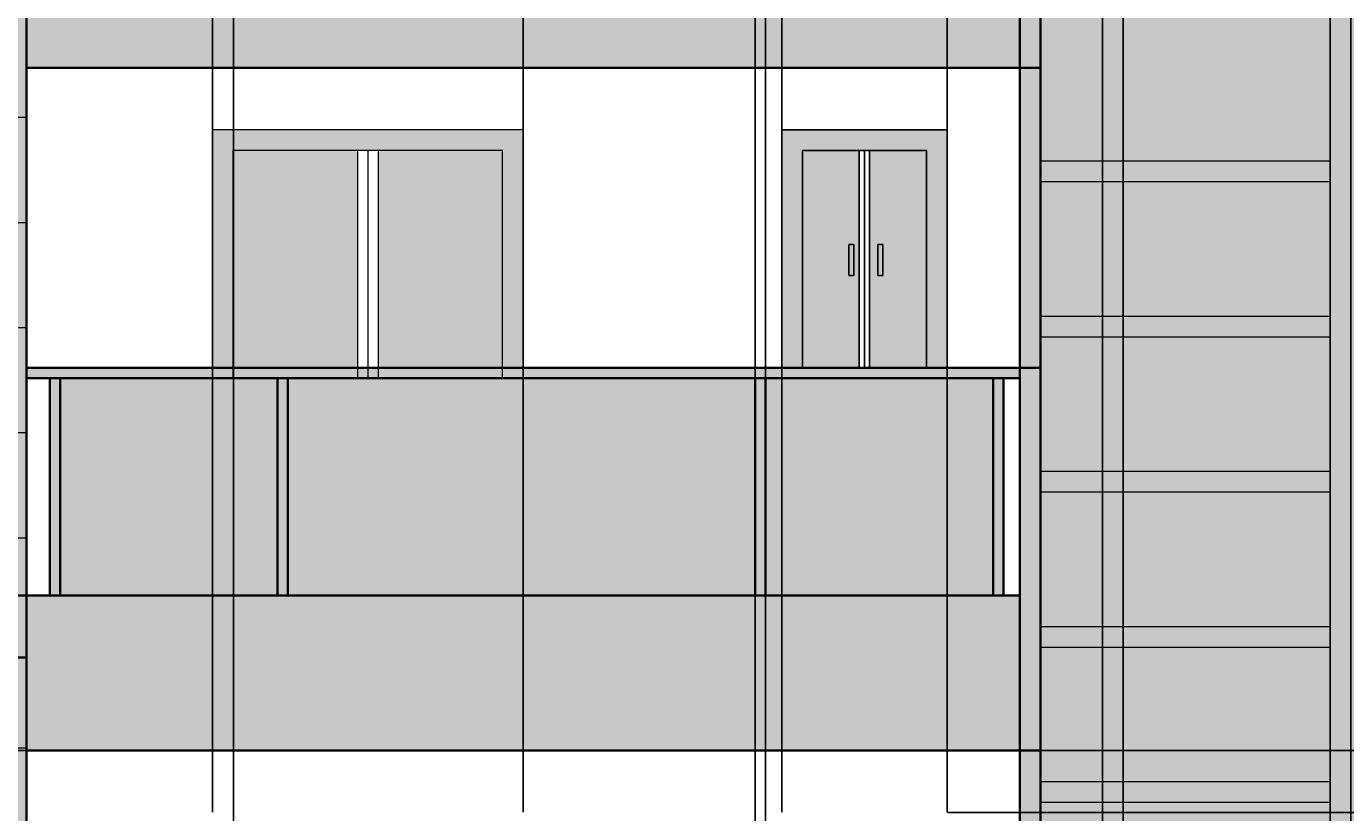
# Model space of a CAD drawing. Units: inches. Extents: x 2794 to 3619, y 522 to 1397.
# Tile 4 of 10: x 2954 to 3209, y 821 to 973. Entities that reach past the tile are written whole.
import ezdxf

# ---------------------------------------------------------------- set-up
doc = ezdxf.new("R2010")
doc.units = ezdxf.units.IN
for name, color, linetype, lineweight in [('A-ANNO-DIMS', 2, 'Continuous', 18), ('A-DOOR', 3, 'Continuous', 25), ('A-ELEV', 7, 'Continuous', 35), ('A-ELEV-PATT', 8, 'Continuous', 13), ('A-GLAZ', 4, 'Continuous', 18)]:
    doc.layers.add(name, color=color, linetype=linetype, lineweight=lineweight)
doc.styles.get("Standard").update_dxf_attribs({"font": 'arial.ttf'})
doc.dimstyles.get("Standard").update_dxf_attribs({"dimtxt": 0.18, "dimasz": 0.18, "dimexe": 0.18, "dimexo": 0.0625, "dimgap": 0.09, "dimtad": 0, "dimtih": 1, "dimtoh": 1, "dimdec": 4, "dimzin": 0, "dimdsep": 46, "dimtxsty": 'Standard', "dimcen": 0.09, "dimadec": 0, "dimazin": 0, "dimtfac": 1, "dimtdec": 4, "dimtofl": 0, "dimtmove": 0, "dimatfit": 3, "dimfxl": 1, "dimtolj": 1, "dimtzin": 0, "dimarcsym": 0})

# ---------------------------------------------------------------- blocks, each defined once
blk = doc.blocks.new('WIN-1500')
at = {"transparency": 33554646}
h = blk.add_hatch(color=256, dxfattribs=at)
h.dxf.hatch_style = 1
h.paths.add_polyline_path([(60, 48), (0, 48), (0, 2), (4, 2), (4, 44), (56, 44), (56, 2), (60, 2)])
at = {"transparency": 33554687}
h = blk.add_hatch(color=256, dxfattribs=at)
h.dxf.hatch_style = 1
h.set_gradient(color1=(248, 246, 176), color2=(74, 13, 14), name='INVCYLINDER')
h.paths.add_polyline_path([(56, 44), (32, 44), (32, 2), (56, 2)])
h.paths.add_polyline_path([(28, 44), (4, 44), (4, 2), (28, 2)])
for p, q in [((0, 0), (0, 48)), ((60, 48), (0, 48)), ((60, 0), (60, 48)), ((56, 44), (4, 44)), ((4, 0), (4, 44)), ((28, 44), (28, 0)), ((30, 44), (30, 0)), ((32, 44), (32, 0)), ((56, 0), (56, 44))]:
    blk.add_line(p, q)
blk = doc.blocks.new('DOOR-BALCONY-DBL')
at = {"transparency": 33554628}
h = blk.add_hatch(color=256, dxfattribs=at)
h.dxf.hatch_style = 1
h.paths.add_polyline_path([(4, 42), (28, 42), (28, 0), (32, 0), (32, 46), (0, 46), (0, 0), (4, 0)])
at = {"transparency": 33554646}
h = blk.add_hatch(color=256, dxfattribs=at)
h.dxf.hatch_style = 1
h.set_gradient(color1=(255, 255, 255), color2=(147, 149, 152), name='INVCYLINDER')
h.paths.add_polyline_path([(15, 42), (4, 42), (4, 0), (15, 0)])
h = blk.add_hatch(color=256, dxfattribs=at)
h.dxf.hatch_style = 1
h.set_gradient(color1=(255, 255, 255), color2=(147, 149, 152), name='INVCYLINDER')
h.paths.add_polyline_path([(28, 42), (17, 42), (17, 0), (28, 0)])
for p, q in [((0, 0), (0, 46)), ((0, 46), (32, 46)), ((4, 46), (28, 46)), ((32, 0), (32, 46)), ((4, 0), (4, 42)), ((4, 42), (28, 42)), ((15, 0), (15, 42)), ((16, 0), (16, 42)), ((17, 0), (17, 42)), ((28, 0), (28, 42))]:
    blk.add_line(p, q)
for points in [[(12.99, 23.83), (13.93, 23.83), (13.93, 17.87), (12.99, 17.87)], [(18.59, 23.83), (19.53, 23.83), (19.53, 17.87), (18.59, 17.87)]]:
    blk.add_lwpolyline(points, close=True)
blk = doc.blocks.new('*D16')
at = {"layer": 'A-ANNO-DIMS', "color": 0, "lineweight": -2, "transparency": 16777216}
for p, q in [((3142.2, 1356.64), (2793.99, 1356.64)), ((2794.17, 1356.46), (2794.17, 959.82)), ((2794.17, 562.82), (2794.17, 959.45)), ((2834.2, 562.64), (2793.99, 562.64))]:
    blk.add_line(p, q, dxfattribs=at)
at = {"layer": 'A-ANNO-DIMS', "color": 0, "transparency": 16777216}
for points in [[(2794.14, 1356.46), (2794.2, 1356.46), (2794.17, 1356.64)], [(2794.14, 562.82), (2794.2, 562.82), (2794.17, 562.64)]]:
    blk.add_solid(points, dxfattribs=at)
at = {"layer": 'Defpoints', "color": 0, "transparency": 16777216}
for p in [(2794.17, 1356.64), (3142.27, 1356.64), (2834.27, 562.64)]:
    blk.add_point(p, dxfattribs=at)
at = {"layer": 'A-ANNO-DIMS', "color": 0, "transparency": 16777216, "insert": (2794.17, 959.64), "char_height": 0.18, "attachment_point": 5}
blk.add_mtext('\\A1;794', dxfattribs=at)
blk = doc.blocks.new('*D28')
at = {"layer": 'A-ANNO-DIMS', "color": 0, "lineweight": -2, "transparency": 16777216}
for p, q in [((2954.27, 832.7), (2954.27, 1396.92)), ((2954.45, 1396.74), (2972.05, 1396.74)), ((2990.09, 1396.74), (2972.48, 1396.74)), ((2990.27, 820.7), (2990.27, 1396.92))]:
    blk.add_line(p, q, dxfattribs=at)
at = {"layer": 'A-ANNO-DIMS', "color": 0, "transparency": 16777216}
for points in [[(2954.45, 1396.77), (2954.45, 1396.71), (2954.27, 1396.74)], [(2990.09, 1396.77), (2990.09, 1396.71), (2990.27, 1396.74)]]:
    blk.add_solid(points, dxfattribs=at)
at = {"layer": 'Defpoints', "color": 0, "transparency": 16777216}
for p in [(2990.27, 1396.74), (2954.27, 832.64), (2990.27, 820.64)]:
    blk.add_point(p, dxfattribs=at)
at = {"layer": 'A-ANNO-DIMS', "color": 0, "transparency": 16777216, "insert": (2972.27, 1396.74), "char_height": 0.18, "attachment_point": 5}
blk.add_mtext('\\A1;36', dxfattribs=at)
blk = doc.blocks.new('*D29')
at = {"layer": 'A-ANNO-DIMS', "color": 0, "lineweight": -2, "transparency": 16777216}
for p, q in [((2990.27, 820.7), (2990.27, 1396.92)), ((2990.45, 1396.74), (2992.11, 1396.74)), ((2994.09, 1396.74), (2992.42, 1396.74)), ((2994.27, 816.7), (2994.27, 1396.92))]:
    blk.add_line(p, q, dxfattribs=at)
at = {"layer": 'A-ANNO-DIMS', "color": 0, "transparency": 16777216}
for points in [[(2990.45, 1396.77), (2990.45, 1396.71), (2990.27, 1396.74)], [(2994.09, 1396.77), (2994.09, 1396.71), (2994.27, 1396.74)]]:
    blk.add_solid(points, dxfattribs=at)
at = {"layer": 'Defpoints', "color": 0, "transparency": 16777216}
for p in [(2994.27, 1396.74), (2990.27, 820.64), (2994.27, 816.64)]:
    blk.add_point(p, dxfattribs=at)
at = {"layer": 'A-ANNO-DIMS', "color": 0, "transparency": 16777216, "insert": (2992.27, 1396.74), "char_height": 0.18, "attachment_point": 5}
blk.add_mtext('\\A1;4', dxfattribs=at)
blk = doc.blocks.new('*D30')
at = {"layer": 'A-ANNO-DIMS', "color": 0, "lineweight": -2, "transparency": 16777216}
for p, q in [((3050.27, 820.7), (3050.27, 1396.92)), ((3050.45, 1396.74), (3075.05, 1396.74)), ((3100.09, 1396.74), (3075.48, 1396.74)), ((3100.27, 820.7), (3100.27, 1396.92))]:
    blk.add_line(p, q, dxfattribs=at)
at = {"layer": 'A-ANNO-DIMS', "color": 0, "transparency": 16777216}
for points in [[(3050.45, 1396.77), (3050.45, 1396.71), (3050.27, 1396.74)], [(3100.09, 1396.77), (3100.09, 1396.71), (3100.27, 1396.74)]]:
    blk.add_solid(points, dxfattribs=at)
at = {"layer": 'Defpoints', "color": 0, "transparency": 16777216}
for p in [(3100.27, 1396.74), (3050.27, 820.64), (3100.27, 820.64)]:
    blk.add_point(p, dxfattribs=at)
at = {"layer": 'A-ANNO-DIMS', "color": 0, "transparency": 16777216, "insert": (3075.27, 1396.74), "char_height": 0.18, "attachment_point": 5}
blk.add_mtext('\\A1;50', dxfattribs=at)
blk = doc.blocks.new('*D31')
at = {"layer": 'A-ANNO-DIMS', "color": 0, "lineweight": -2, "transparency": 16777216}
for p, q in [((3132.27, 820.7), (3132.27, 1396.92)), ((3132.45, 1396.74), (3139.06, 1396.74)), ((3146.09, 1396.74), (3139.48, 1396.74)), ((3146.27, 774.7), (3146.27, 1396.92))]:
    blk.add_line(p, q, dxfattribs=at)
at = {"layer": 'A-ANNO-DIMS', "color": 0, "transparency": 16777216}
for points in [[(3132.45, 1396.77), (3132.45, 1396.71), (3132.27, 1396.74)], [(3146.09, 1396.77), (3146.09, 1396.71), (3146.27, 1396.74)]]:
    blk.add_solid(points, dxfattribs=at)
at = {"layer": 'Defpoints', "color": 0, "transparency": 16777216}
for p in [(3146.27, 1396.74), (3132.27, 820.64), (3146.27, 774.64)]:
    blk.add_point(p, dxfattribs=at)
at = {"layer": 'A-ANNO-DIMS', "color": 0, "transparency": 16777216, "insert": (3139.27, 1396.74), "char_height": 0.18, "attachment_point": 5}
blk.add_mtext('\\A1;14', dxfattribs=at)
blk = doc.blocks.new('*D37')
at = {"layer": 'A-ANNO-DIMS', "color": 0, "lineweight": -2, "transparency": 16777216}
for p, q in [((3095.13, 772.7), (3095.13, 1396.92)), ((3095.31, 1396.74), (3095.98, 1396.74)), ((3096.95, 1396.74), (3096.28, 1396.74)), ((3097.13, 772.7), (3097.13, 1396.92))]:
    blk.add_line(p, q, dxfattribs=at)
at = {"layer": 'A-ANNO-DIMS', "color": 0, "transparency": 16777216}
for points in [[(3095.31, 1396.77), (3095.31, 1396.71), (3095.13, 1396.74)], [(3096.95, 1396.77), (3096.95, 1396.71), (3097.13, 1396.74)]]:
    blk.add_solid(points, dxfattribs=at)
at = {"layer": 'Defpoints', "color": 0, "transparency": 16777216}
for p in [(3097.13, 1396.74), (3095.13, 772.64), (3097.13, 772.64)]:
    blk.add_point(p, dxfattribs=at)
at = {"layer": 'A-ANNO-DIMS', "color": 0, "transparency": 16777216, "insert": (3096.13, 1396.74), "char_height": 0.18, "attachment_point": 5}
blk.add_mtext('\\A1;2', dxfattribs=at)
blk = doc.blocks.new('*D42')
at = {"layer": 'A-ANNO-DIMS', "color": 0, "lineweight": -2, "transparency": 16777216}
for p, q in [((2958.76, 862.64), (2793.99, 862.64)), ((2794.17, 862.46), (2794.17, 847.82)), ((2794.17, 832.82), (2794.17, 847.45)), ((2954.2, 832.64), (2793.99, 832.64))]:
    blk.add_line(p, q, dxfattribs=at)
at = {"layer": 'A-ANNO-DIMS', "color": 0, "transparency": 16777216}
for points in [[(2794.14, 862.46), (2794.2, 862.46), (2794.17, 862.64)], [(2794.14, 832.82), (2794.2, 832.82), (2794.17, 832.64)]]:
    blk.add_solid(points, dxfattribs=at)
at = {"layer": 'Defpoints', "color": 0, "transparency": 16777216}
for p in [(2794.17, 862.64), (2958.83, 862.64), (2954.27, 832.64)]:
    blk.add_point(p, dxfattribs=at)
at = {"layer": 'A-ANNO-DIMS', "color": 0, "transparency": 16777216, "insert": (2794.17, 847.64), "char_height": 0.18, "attachment_point": 5}
blk.add_mtext('\\A1;30', dxfattribs=at)
blk = doc.blocks.new('*D43')
at = {"layer": 'A-ANNO-DIMS', "color": 0, "lineweight": -2, "transparency": 16777216}
for p, q in [((3150.33, 832.64), (3618.55, 832.64)), ((3618.37, 832.46), (3618.37, 826.82)), ((3618.37, 820.82), (3618.37, 826.45)), ((3132.33, 820.64), (3618.55, 820.64))]:
    blk.add_line(p, q, dxfattribs=at)
at = {"layer": 'A-ANNO-DIMS', "color": 0, "transparency": 16777216}
for points in [[(3618.34, 832.46), (3618.4, 832.46), (3618.37, 832.64)], [(3618.34, 820.82), (3618.4, 820.82), (3618.37, 820.64)]]:
    blk.add_solid(points, dxfattribs=at)
at = {"layer": 'Defpoints', "color": 0, "transparency": 16777216}
for p in [(3150.27, 832.64), (3618.37, 832.64), (3132.27, 820.64)]:
    blk.add_point(p, dxfattribs=at)
at = {"layer": 'A-ANNO-DIMS', "color": 0, "transparency": 16777216, "insert": (3618.37, 826.64), "char_height": 0.18, "attachment_point": 5}
blk.add_mtext('\\A1;12', dxfattribs=at)
blk = doc.blocks.new('*D49')
at = {"layer": 'A-ANNO-DIMS', "color": 0, "lineweight": -2, "transparency": 16777216}
for p, q in [((3146.27, 1256.19), (3146.27, 522.36)), ((3150.27, 1254.57), (3150.27, 522.36)), ((3146.45, 522.54), (3148.11, 522.54)), ((3150.09, 522.54), (3148.42, 522.54))]:
    blk.add_line(p, q, dxfattribs=at)
at = {"layer": 'A-ANNO-DIMS', "color": 0, "transparency": 16777216}
for points in [[(3146.45, 522.57), (3146.45, 522.51), (3146.27, 522.54)], [(3150.09, 522.57), (3150.09, 522.51), (3150.27, 522.54)]]:
    blk.add_solid(points, dxfattribs=at)
at = {"layer": 'Defpoints', "color": 0, "transparency": 16777216}
for p in [(3146.27, 1256.25), (3150.27, 1254.64), (3150.27, 522.54)]:
    blk.add_point(p, dxfattribs=at)
at = {"layer": 'A-ANNO-DIMS', "color": 0, "transparency": 16777216, "insert": (3148.27, 522.54), "char_height": 0.18, "attachment_point": 5}
blk.add_mtext('\\A1;4', dxfattribs=at)
blk = doc.blocks.new('*D50')
at = {"layer": 'A-ANNO-DIMS', "color": 0, "lineweight": -2, "transparency": 16777216}
for p, q in [((3150.27, 1254.57), (3150.27, 522.36)), ((3206.27, 1254.57), (3206.27, 522.36)), ((3150.45, 522.54), (3178.05, 522.54)), ((3206.09, 522.54), (3178.48, 522.54))]:
    blk.add_line(p, q, dxfattribs=at)
at = {"layer": 'A-ANNO-DIMS', "color": 0, "transparency": 16777216}
for points in [[(3150.45, 522.57), (3150.45, 522.51), (3150.27, 522.54)], [(3206.09, 522.57), (3206.09, 522.51), (3206.27, 522.54)]]:
    blk.add_solid(points, dxfattribs=at)
at = {"layer": 'Defpoints', "color": 0, "transparency": 16777216}
for p in [(3150.27, 1254.64), (3206.27, 1254.64), (3206.27, 522.54)]:
    blk.add_point(p, dxfattribs=at)
at = {"layer": 'A-ANNO-DIMS', "color": 0, "transparency": 16777216, "insert": (3178.27, 522.54), "char_height": 0.18, "attachment_point": 5}
blk.add_mtext('\\A1;56', dxfattribs=at)
blk = doc.blocks.new('*D51')
at = {"layer": 'A-ANNO-DIMS', "color": 0, "lineweight": -2, "transparency": 16777216}
for p, q in [((3206.27, 1254.57), (3206.27, 522.36)), ((3210.27, 1254.57), (3210.27, 522.36)), ((3206.45, 522.54), (3208.11, 522.54)), ((3210.09, 522.54), (3208.42, 522.54))]:
    blk.add_line(p, q, dxfattribs=at)
at = {"layer": 'A-ANNO-DIMS', "color": 0, "transparency": 16777216}
for points in [[(3206.45, 522.57), (3206.45, 522.51), (3206.27, 522.54)], [(3210.09, 522.57), (3210.09, 522.51), (3210.27, 522.54)]]:
    blk.add_solid(points, dxfattribs=at)
at = {"layer": 'Defpoints', "color": 0, "transparency": 16777216}
for p in [(3206.27, 1254.64), (3210.27, 1254.64), (3210.27, 522.54)]:
    blk.add_point(p, dxfattribs=at)
at = {"layer": 'A-ANNO-DIMS', "color": 0, "transparency": 16777216, "insert": (3208.27, 522.54), "char_height": 0.18, "attachment_point": 5}
blk.add_mtext('\\A1;4', dxfattribs=at)
blk = doc.blocks.new('*D56')
at = {"layer": 'A-ANNO-DIMS', "color": 0, "lineweight": -2, "transparency": 16777216}
for p, q in [((3162.27, 664.7), (3162.27, 1396.92)), ((3162.45, 1396.74), (3206.05, 1396.74)), ((3250.09, 1396.74), (3206.49, 1396.74)), ((3250.27, 664.7), (3250.27, 1396.92))]:
    blk.add_line(p, q, dxfattribs=at)
at = {"layer": 'A-ANNO-DIMS', "color": 0, "transparency": 16777216}
for points in [[(3162.45, 1396.77), (3162.45, 1396.71), (3162.27, 1396.74)], [(3250.09, 1396.77), (3250.09, 1396.71), (3250.27, 1396.74)]]:
    blk.add_solid(points, dxfattribs=at)
at = {"layer": 'Defpoints', "color": 0, "transparency": 16777216}
for p in [(3250.27, 1396.74), (3162.27, 664.64), (3250.27, 664.64)]:
    blk.add_point(p, dxfattribs=at)
at = {"layer": 'A-ANNO-DIMS', "color": 0, "transparency": 16777216, "insert": (3206.27, 1396.74), "char_height": 0.18, "attachment_point": 5}
blk.add_mtext('\\A1;88', dxfattribs=at)
blk = doc.blocks.new('*D57')
at = {"layer": 'A-ANNO-DIMS', "color": 0, "lineweight": -2, "transparency": 16777216}
for p, q in [((3162.27, 664.7), (3162.27, 1396.92)), ((3162.45, 1396.74), (3164.11, 1396.74)), ((3166.09, 1396.74), (3164.42, 1396.74)), ((3166.27, 660.7), (3166.27, 1396.92))]:
    blk.add_line(p, q, dxfattribs=at)
at = {"layer": 'A-ANNO-DIMS', "color": 0, "transparency": 16777216}
for points in [[(3162.45, 1396.77), (3162.45, 1396.71), (3162.27, 1396.74)], [(3166.09, 1396.77), (3166.09, 1396.71), (3166.27, 1396.74)]]:
    blk.add_solid(points, dxfattribs=at)
at = {"layer": 'Defpoints', "color": 0, "transparency": 16777216}
for p in [(3166.27, 1396.74), (3162.27, 664.64), (3166.27, 660.64)]:
    blk.add_point(p, dxfattribs=at)
at = {"layer": 'A-ANNO-DIMS', "color": 0, "transparency": 16777216, "insert": (3164.27, 1396.74), "char_height": 0.18, "attachment_point": 5}
blk.add_mtext('\\A1;4', dxfattribs=at)
blk = doc.blocks.new('*D58')
at = {"layer": 'A-ANNO-DIMS', "color": 0, "lineweight": -2, "transparency": 16777216}
for p, q in [((3150.27, 580.7), (3150.27, 1396.92)), ((3150.45, 1396.74), (3156.06, 1396.74)), ((3162.09, 1396.74), (3156.48, 1396.74)), ((3162.27, 664.7), (3162.27, 1396.92))]:
    blk.add_line(p, q, dxfattribs=at)
at = {"layer": 'A-ANNO-DIMS', "color": 0, "transparency": 16777216}
for points in [[(3150.45, 1396.77), (3150.45, 1396.71), (3150.27, 1396.74)], [(3162.09, 1396.77), (3162.09, 1396.71), (3162.27, 1396.74)]]:
    blk.add_solid(points, dxfattribs=at)
at = {"layer": 'Defpoints', "color": 0, "transparency": 16777216}
for p in [(3162.27, 1396.74), (3162.27, 664.64), (3150.27, 580.64)]:
    blk.add_point(p, dxfattribs=at)
at = {"layer": 'A-ANNO-DIMS', "color": 0, "transparency": 16777216, "insert": (3156.27, 1396.74), "char_height": 0.18, "attachment_point": 5}
blk.add_mtext('\\A1;12', dxfattribs=at)

msp = doc.modelspace()

# ---------------------------------------------------------------- hatches: boundary and pattern name
at = {"layer": 'A-ELEV-PATT', "transparency": 33554687}
h = msp.add_hatch(color=256, dxfattribs=at)
h.dxf.hatch_style = 1
h.paths.add_polyline_path([(3262.2659, 1350.6351), (3150.2659, 1350.6351), (3150.2659, 1279.0155, -0.68639605), (3262.2659, 1279.0155)])
h.paths.add_polyline_path([(3210.2659, 1314.1121), (3210.2659, 1258.6351), (3262.2659, 1258.6351, 0.39146256)])
h.paths.add_polyline_path([(3206.2659, 1314.2551, 0.41222069), (3150.2659, 1258.6351), (3206.2659, 1258.6351)])
h.paths.add_polyline_path([(3262.2659, 1254.6351), (3210.2659, 1254.6351), (3210.2659, 1216.6351), (3262.2659, 1216.6351)])
h.paths.add_polyline_path([(3206.2659, 1254.6351), (3150.2659, 1254.6351), (3150.2659, 1216.6351), (3206.2659, 1216.6351)])
h.paths.add_polyline_path([(3262.2659, 1212.6351), (3210.2659, 1212.6351), (3210.2659, 1186.6351), (3262.2659, 1186.6351)])
h.paths.add_polyline_path([(3206.2659, 1212.6351), (3150.2659, 1212.6351), (3150.2659, 1186.6351), (3206.2659, 1186.6351)])
h.paths.add_polyline_path([(3206.2659, 1182.6351), (3150.2659, 1182.6351), (3150.2659, 1156.6351), (3206.2659, 1156.6351)])
h.paths.add_polyline_path([(3262.2659, 1182.6351), (3210.2659, 1182.6351), (3210.2659, 1156.6351), (3262.2659, 1156.6351)])
h.paths.add_polyline_path([(3262.2659, 1152.6351), (3210.2659, 1152.6351), (3210.2659, 1126.6351), (3262.2659, 1126.6351)])
h.paths.add_polyline_path([(3206.2659, 1152.6351), (3150.2659, 1152.6351), (3150.2659, 1126.6351), (3206.2659, 1126.6351)])
h.paths.add_polyline_path([(3262.2659, 1122.6351), (3210.2659, 1122.6351), (3210.2659, 1096.6351), (3262.2659, 1096.6351)])
h.paths.add_polyline_path([(3206.2659, 1122.6351), (3150.2659, 1122.6351), (3150.2659, 1096.6351), (3206.2659, 1096.6351)])
h.paths.add_polyline_path([(3206.2659, 1092.6351), (3150.2659, 1092.6351), (3150.2659, 1066.6351), (3206.2659, 1066.6351)])
h.paths.add_polyline_path([(3262.2659, 1092.6351), (3210.2659, 1092.6351), (3210.2659, 1066.6351), (3262.2659, 1066.6351)])
h.paths.add_polyline_path([(3262.2659, 1062.6351), (3210.2659, 1062.6351), (3210.2659, 1036.6351), (3262.2659, 1036.6351)])
h.paths.add_polyline_path([(3206.2659, 1062.6351), (3150.2659, 1062.6351), (3150.2659, 1036.6351), (3206.2659, 1036.6351)])
h.paths.add_polyline_path([(3206.2659, 1032.6351), (3150.2659, 1032.6351), (3150.2659, 1006.6351), (3206.2659, 1006.6351)])
h.paths.add_polyline_path([(3262.2659, 1032.6351), (3210.2659, 1032.6351), (3210.2659, 1006.6351), (3262.2659, 1006.6351)])
h.paths.add_polyline_path([(3262.2659, 1002.6351), (3210.2659, 1002.6351), (3210.2659, 976.6351), (3262.2659, 976.6351)])
h.paths.add_polyline_path([(3206.2659, 1002.6351), (3150.2659, 1002.6351), (3150.2659, 976.6351), (3206.2659, 976.6351)])
h.paths.add_polyline_path([(3206.2659, 972.6351), (3150.2659, 972.6351), (3150.2659, 946.6351), (3206.2659, 946.6351)])
h.paths.add_polyline_path([(3206.2659, 942.6351), (3150.2659, 942.6351), (3150.2659, 916.6351), (3206.2659, 916.6351)])
h.paths.add_polyline_path([(3262.2659, 942.6351), (3210.2659, 942.6351), (3210.2659, 916.6351), (3262.2659, 916.6351)])
h.paths.add_polyline_path([(3262.2659, 972.6351), (3210.2659, 972.6351), (3210.2659, 946.6351), (3262.2659, 946.6351)])
h.paths.add_polyline_path([(3262.2659, 912.6351), (3210.2659, 912.6351), (3210.2659, 886.6351), (3262.2659, 886.6351)])
h.paths.add_polyline_path([(3206.2659, 912.6351), (3150.2659, 912.6351), (3150.2659, 886.6351), (3206.2659, 886.6351)])
h.paths.add_polyline_path([(3206.2659, 882.6351), (3150.2659, 882.6351), (3150.2659, 856.6351), (3206.2659, 856.6351)])
h.paths.add_polyline_path([(3262.2659, 882.6351), (3210.2659, 882.6351), (3210.2659, 856.6351), (3262.2659, 856.6351)])
h.paths.add_polyline_path([(3262.2659, 852.6351), (3210.2659, 852.6351), (3210.2659, 826.6351), (3262.2659, 826.6351)])
h.paths.add_polyline_path([(3206.2659, 852.6351), (3150.2659, 852.6351), (3150.2659, 826.6351), (3206.2659, 826.6351)])
h.paths.add_polyline_path([(3206.2659, 822.6351), (3150.2659, 822.6351), (3150.2659, 796.6351), (3206.2659, 796.6351)])
h.paths.add_polyline_path([(3262.2659, 822.6351), (3210.2659, 822.6351), (3210.2659, 796.6351), (3262.2659, 796.6351)])
h.paths.add_polyline_path([(3262.2659, 792.6351), (3210.2659, 792.6351), (3210.2659, 766.6351), (3262.2659, 766.6351)])
h.paths.add_polyline_path([(3206.2659, 792.6351), (3150.2659, 792.6351), (3150.2659, 766.6351), (3206.2659, 766.6351)])
h.paths.add_polyline_path([(3206.2659, 762.6351), (3150.2659, 762.6351), (3150.2659, 736.6351), (3206.2659, 736.6351)])
h.paths.add_polyline_path([(3206.2659, 732.6351), (3150.2659, 732.6351), (3150.2659, 706.6351), (3206.2659, 706.6351)])
h.paths.add_polyline_path([(3262.2659, 732.6351), (3210.2659, 732.6351), (3210.2659, 706.6351), (3262.2659, 706.6351)])
h.paths.add_polyline_path([(3262.2659, 762.6351), (3210.2659, 762.6351), (3210.2659, 736.6351), (3262.2659, 736.6351)])
h = msp.add_hatch(color=256, dxfattribs=at)
h.dxf.hatch_style = 1
h.paths.add_polyline_path([(3150.2659, 1257.8725, -0.00340445), (3150.2659, 1258.6351), (3146.2659, 1258.6351), (3146.2659, 1228.6351), (3150.2659, 1228.6351)])
h.paths.add_polyline_path([(3262.2659, 1258.6351), (3210.2659, 1258.6351), (3210.2659, 1314.1121, 0.01787385), (3206.2659, 1314.2551), (3206.2659, 1258.6351), (3150.2659, 1258.6351), (3150.2659, 1254.6351), (3206.2659, 1254.6351), (3206.2659, 1216.6351), (3150.2659, 1216.6351), (3150.2659, 1212.6351), (3206.2659, 1212.6351), (3206.2659, 1186.6351), (3150.2659, 1186.6351), (3150.2659, 1182.6351), (3206.2659, 1182.6351), (3206.2659, 1156.6351), (3150.2659, 1156.6351), (3150.2659, 1152.6351), (3206.2659, 1152.6351), (3206.2659, 1126.6351), (3150.2659, 1126.6351), (3150.2659, 1122.6351), (3206.2659, 1122.6351), (3206.2659, 1096.6351), (3150.2659, 1096.6351), (3150.2659, 1092.6351), (3206.2659, 1092.6351), (3206.2659, 1066.6351), (3150.2659, 1066.6351), (3150.2659, 1062.6351), (3206.2659, 1062.6351), (3206.2659, 1036.6351), (3150.2659, 1036.6351), (3150.2659, 1032.6351), (3206.2659, 1032.6351), (3206.2659, 1006.6351), (3150.2659, 1006.6351), (3150.2659, 1002.6351), (3206.2659, 1002.6351), (3206.2659, 976.6351), (3150.2659, 976.6351), (3150.2659, 972.6351), (3206.2659, 972.6351), (3206.2659, 946.6351), (3150.2659, 946.6351), (3150.2659, 942.6351), (3206.2659, 942.6351), (3206.2659, 916.6351), (3150.2659, 916.6351), (3150.2659, 912.6351), (3206.2659, 912.6351), (3206.2659, 886.6351), (3150.2659, 886.6351), (3150.2659, 882.6351), (3206.2659, 882.6351), (3206.2659, 856.6351), (3150.2659, 856.6351), (3150.2659, 852.6351), (3206.2659, 852.6351), (3206.2659, 826.6351), (3150.2659, 826.6351), (3150.2659, 822.6351), (3206.2659, 822.6351), (3206.2659, 796.6351), (3150.2659, 796.6351), (3150.2659, 792.6351), (3206.2659, 792.6351), (3206.2659, 766.6351), (3150.2659, 766.6351), (3150.2659, 762.6351), (3206.2659, 762.6351), (3206.2659, 736.6351), (3150.2659, 736.6351), (3150.2659, 732.6351), (3206.2659, 732.6351), (3206.2659, 706.6351), (3150.2659, 706.6351), (3150.2659, 702.6351), (3262.2659, 702.6351), (3262.2659, 706.6351), (3210.2659, 706.6351), (3210.2659, 732.6351), (3262.2659, 732.6351), (3262.2659, 736.6351), (3210.2659, 736.6351), (3210.2659, 762.6351), (3262.2659, 762.6351), (3262.2659, 766.6351), (3210.2659, 766.6351), (3210.2659, 792.6351), (3262.2659, 792.6351), (3262.2659, 796.6351), (3210.2659, 796.6351), (3210.2659, 822.6351), (3262.2659, 822.6351), (3262.2659, 826.6351), (3210.2659, 826.6351), (3210.2659, 852.6351), (3262.2659, 852.6351), (3262.2659, 856.6351), (3210.2659, 856.6351), (3210.2659, 882.6351), (3262.2659, 882.6351), (3262.2659, 886.6351), (3210.2659, 886.6351), (3210.2659, 912.6351), (3262.2659, 912.6351), (3262.2659, 916.6351), (3210.2659, 916.6351), (3210.2659, 942.6351), (3262.2659, 942.6351), (3262.2659, 946.6351), (3210.2659, 946.6351), (3210.2659, 972.6351), (3262.2659, 972.6351), (3262.2659, 976.6351), (3210.2659, 976.6351), (3210.2659, 1002.6351), (3262.2659, 1002.6351), (3262.2659, 1006.6351), (3210.2659, 1006.6351), (3210.2659, 1032.6351), (3262.2659, 1032.6351), (3262.2659, 1036.6351), (3210.2659, 1036.6351), (3210.2659, 1062.6351), (3262.2659, 1062.6351), (3262.2659, 1066.6351), (3210.2659, 1066.6351), (3210.2659, 1092.6351), (3262.2659, 1092.6351), (3262.2659, 1096.6351), (3210.2659, 1096.6351), (3210.2659, 1122.6351), (3262.2659, 1122.6351), (3262.2659, 1126.6351), (3210.2659, 1126.6351), (3210.2659, 1152.6351), (3262.2659, 1152.6351), (3262.2659, 1156.6351), (3210.2659, 1156.6351), (3210.2659, 1182.6351), (3262.2659, 1182.6351), (3262.2659, 1186.6351), (3210.2659, 1186.6351), (3210.2659, 1212.6351), (3262.2659, 1212.6351), (3262.2659, 1216.6351), (3210.2659, 1216.6351), (3210.2659, 1254.6351), (3262.2659, 1254.6351)])
h = msp.add_hatch(color=256, dxfattribs=at)
h.dxf.hatch_style = 1
h.paths.add_polyline_path([(2852.2659, 1246.6351), (2954.2659, 1246.6351), (2954.2659, 1258.6351), (2900.2659, 1258.6351), (2900.2659, 1294.6351), (2852.2659, 1294.6351)])
h.paths.add_polyline_path([(3512.2659, 1294.6351), (3512.2659, 1258.6351), (3458.2659, 1258.6351), (3458.2659, 1246.6351), (3560.2659, 1246.6351), (3560.2659, 1294.6351)])
h.paths.add_polyline_path([(2954.2659, 1114.6351), (2954.2659, 1126.6351), (2852.2659, 1126.6351), (2852.2659, 1114.6351)])
h.paths.add_polyline_path([(3560.2659, 1114.6351), (3560.2659, 1126.6351), (3458.2659, 1126.6351), (3458.2659, 1114.6351)])
h.paths.add_polyline_path([(3560.2659, 982.6351), (3560.2659, 994.6351), (3458.2659, 994.6351), (3458.2659, 982.6351)])
h.paths.add_polyline_path([(2954.2659, 982.6351), (2954.2659, 994.6351), (2852.2659, 994.6351), (2852.2659, 982.6351)])
h.paths.add_polyline_path([(2852.2659, 862.6351), (2852.2659, 850.6351), (2954.2659, 850.6351), (2954.2659, 862.6351)])
h.paths.add_polyline_path([(2852.2659, 730.6351), (2852.2659, 718.6351), (2954.2659, 718.6351), (2954.2659, 730.6351)])
h.paths.add_polyline_path([(3560.2659, 718.6351), (3560.2659, 730.6351), (3458.2659, 730.6351), (3458.2659, 718.6351)])
h.paths.add_polyline_path([(3560.2659, 850.6351), (3560.2659, 862.6351), (3458.2659, 862.6351), (3458.2659, 850.6351)])
h = msp.add_hatch(color=256, dxfattribs=at)
h.dxf.hatch_style = 1
h.paths.add_polyline_path([(3146.2659, 1096.6351), (3146.2659, 1126.6351), (2954.2659, 1126.6351), (2954.2659, 1096.6351)])
h.paths.add_polyline_path([(3458.2659, 1096.6351), (3458.2659, 1126.6351), (3266.2659, 1126.6351), (3266.2659, 1096.6351)])
h.paths.add_polyline_path([(3458.2659, 964.6351), (3458.2659, 994.6351), (3266.2659, 994.6351), (3266.2659, 964.6351)])
h.paths.add_polyline_path([(3146.2659, 964.6351), (3146.2659, 994.6351), (2954.2659, 994.6351), (2954.2659, 964.6351)])
h.paths.add_polyline_path([(3458.2659, 832.6351), (3458.2659, 862.6351), (3266.2659, 862.6351), (3266.2659, 832.6351)])
h.paths.add_polyline_path([(3146.2659, 832.6351), (3146.2659, 862.6351), (2954.2659, 862.6351), (2954.2659, 832.6351)])
h.paths.add_polyline_path([(3458.2659, 700.6351), (3458.2659, 730.6351), (3266.2659, 730.6351), (3266.2659, 700.6351)])
h.paths.add_polyline_path([(3146.2659, 700.6351), (3146.2659, 730.6351), (2954.2659, 730.6351), (2954.2659, 700.6351)])
h.paths.add_polyline_path([(3266.2659, 1294.6351), (3266.2659, 1258.6351), (3266.2659, 1228.6351), (3458.2659, 1228.6351), (3458.2659, 1294.6351)])
h.paths.add_polyline_path([(3146.2659, 1228.6351), (3146.2659, 1256.2485, -0.00994307), (3146.2659, 1258.6351), (3146.2659, 1294.6351), (2954.2659, 1294.6351), (2954.2659, 1228.6351)])
at = {"layer": 'A-ELEV-PATT'}
h = msp.add_hatch(dxfattribs=at)
h.set_pattern_fill('AR-B816', color=256, scale=0.1)
h.paths.add_polyline_path([(2954.2659, 1114.6351), (2852.2659, 1114.6351), (2852.2659, 994.6351), (2954.2659, 994.6351)])
h.paths.add_polyline_path([(2954.2659, 1246.6351), (2852.2659, 1246.6351), (2852.2659, 1126.6351), (2954.2659, 1126.6351)])
h.paths.add_polyline_path([(2954.2659, 982.6351), (2852.2659, 982.6351), (2852.2659, 862.6351), (2954.2659, 862.6351)])
h.paths.add_polyline_path([(2954.2659, 850.6351), (2852.2659, 850.6351), (2852.2659, 730.6351), (2954.2659, 730.6351)])
h.paths.add_polyline_path([(3560.2659, 850.6351), (3458.2659, 850.6351), (3458.2659, 730.6351), (3560.2659, 730.6351)])
h.paths.add_polyline_path([(3560.2659, 982.6351), (3458.2659, 982.6351), (3458.2659, 862.6351), (3560.2659, 862.6351)])
h.paths.add_polyline_path([(3560.2659, 1114.6351), (3458.2659, 1114.6351), (3458.2659, 994.6351), (3560.2659, 994.6351)])
h.paths.add_polyline_path([(3560.2659, 1246.6351), (3458.2659, 1246.6351), (3458.2659, 1126.6351), (3560.2659, 1126.6351)])
h.paths.add_polyline_path([(2852.2659, 642.6351), (2954.2659, 642.6351), (2954.2659, 718.6351), (2852.2659, 718.6351)])
h.paths.add_polyline_path([(3458.2659, 640.6351), (3560.2659, 640.6351), (3560.2659, 718.6351), (3458.2659, 718.6351)])
at = {"layer": 'A-ELEV-PATT', "transparency": 33554630}
h = msp.add_hatch(color=256, dxfattribs=at)
h.dxf.hatch_style = 1
h.paths.add_polyline_path([(2954.2659, 1114.6351), (2852.2659, 1114.6351), (2852.2659, 994.6351), (2954.2659, 994.6351)])
h.paths.add_polyline_path([(2954.2659, 982.6351), (2852.2659, 982.6351), (2852.2659, 862.6351), (2954.2659, 862.6351)])
h.paths.add_polyline_path([(2954.2659, 850.6351), (2852.2659, 850.6351), (2852.2659, 730.6351), (2954.2659, 730.6351)])
h.paths.add_polyline_path([(3560.2659, 850.6351), (3458.2659, 850.6351), (3458.2659, 730.6351), (3560.2659, 730.6351)])
h.paths.add_polyline_path([(3560.2659, 982.6351), (3458.2659, 982.6351), (3458.2659, 862.6351), (3560.2659, 862.6351)])
h.paths.add_polyline_path([(3560.2659, 1114.6351), (3458.2659, 1114.6351), (3458.2659, 994.6351), (3560.2659, 994.6351)])
h.paths.add_polyline_path([(3560.2659, 1246.6351), (3458.2659, 1246.6351), (3458.2659, 1126.6351), (3560.2659, 1126.6351)])
h.paths.add_polyline_path([(2852.2659, 642.6351), (2954.2659, 642.6351), (2954.2659, 718.6351), (2852.2659, 718.6351)])
h.paths.add_polyline_path([(3458.2659, 642.6351), (3560.2659, 642.6351), (3560.2659, 718.6351), (3458.2659, 718.6351)])
at = {"layer": 'A-ELEV-PATT', "transparency": 33554687}
h = msp.add_hatch(color=256, dxfattribs=at)
h.dxf.hatch_style = 1
h.paths.add_polyline_path([(3150.2659, 1228.6351), (3146.2659, 1228.6351), (3146.2659, 1126.6351), (3150.2659, 1126.6351)])
h.paths.add_polyline_path([(3150.2659, 1126.6351), (3146.2659, 1126.6351), (3146.2659, 1038.6351), (3150.2659, 1038.6351)])
h.paths.add_polyline_path([(3150.2659, 1038.6351), (3146.2659, 1038.6351), (3146.2659, 964.6351), (3150.2659, 964.6351)])
h.paths.add_polyline_path([(3150.2659, 964.6351), (3146.2659, 964.6351), (3146.2659, 906.6351), (3150.2659, 906.6351)])
h.paths.add_polyline_path([(3150.2659, 906.6351), (3146.2659, 906.6351), (3146.2659, 832.6351), (3150.2659, 832.6351)])
h.paths.add_polyline_path([(3150.2659, 832.6351), (3146.2659, 832.6351), (3146.2659, 730.6351), (3150.2659, 730.6351)])
h = msp.add_hatch(color=256, dxfattribs=at)
h.dxf.hatch_style = 1
h.paths.add_polyline_path([(3097.1329, 904.6351), (3095.1329, 904.6351), (3095.1329, 862.6351), (3097.1329, 862.6351)])
h.paths.add_polyline_path([(3143.112, 904.6351), (3141.112, 904.6351), (3141.112, 862.6351), (3143.112, 862.6351)])
h.paths.add_polyline_path([(3146.2659, 906.6351), (2954.2659, 906.6351), (2954.2659, 904.6351), (3146.2659, 904.6351)])
h.paths.add_polyline_path([(3004.8268, 904.6351), (3002.8268, 904.6351), (3002.8268, 862.6351), (3004.8268, 862.6351)])
h.paths.add_polyline_path([(2960.8268, 904.6351), (2958.8268, 904.6351), (2958.8268, 862.6351), (2960.8268, 862.6351)])
h.paths.add_polyline_path([(3146.2659, 1038.6351), (2954.2659, 1038.6351), (2954.2659, 1036.6351), (3146.2659, 1036.6351)])
h.paths.add_polyline_path([(2960.8268, 1036.6351), (2958.8268, 1036.6351), (2958.8268, 994.6351), (2960.8268, 994.6351)])
h.paths.add_polyline_path([(3004.8268, 1036.6351), (3002.8268, 1036.6351), (3002.8268, 994.6351), (3004.8268, 994.6351)])
h.paths.add_polyline_path([(3143.112, 1036.6351), (3141.112, 1036.6351), (3141.112, 994.6351), (3143.112, 994.6351)])
h.paths.add_polyline_path([(3097.1329, 1036.6351), (3095.1329, 1036.6351), (3095.1329, 994.6351), (3097.1329, 994.6351)])
h.paths.add_polyline_path([(3146.2659, 1170.6351), (2954.2659, 1170.6351), (2954.2659, 1168.6351), (3146.2659, 1168.6351)])
h.paths.add_polyline_path([(3004.8268, 1168.6351), (3002.8268, 1168.6351), (3002.8268, 1126.6351), (3004.8268, 1126.6351)])
h.paths.add_polyline_path([(2960.8268, 1168.6351), (2958.8268, 1168.6351), (2958.8268, 1126.6351), (2960.8268, 1126.6351)])
h.paths.add_polyline_path([(3143.112, 1168.6351), (3141.112, 1168.6351), (3141.112, 1126.6351), (3143.112, 1126.6351)])
h.paths.add_polyline_path([(3097.1329, 1168.6351), (3095.1329, 1168.6351), (3095.1329, 1126.6351), (3097.1329, 1126.6351)])
h.paths.add_polyline_path([(3458.2659, 1170.6351), (3266.2659, 1170.6351), (3266.2659, 1168.6351), (3458.2659, 1168.6351)])
h.paths.add_polyline_path([(3272.407, 1168.6351), (3270.407, 1168.6351), (3270.407, 1126.6351), (3272.407, 1126.6351)])
h.paths.add_polyline_path([(3316.407, 1168.6351), (3314.407, 1168.6351), (3314.407, 1126.6351), (3316.407, 1126.6351)])
h.paths.add_polyline_path([(3408.7131, 1168.6351), (3406.7131, 1168.6351), (3406.7131, 1126.6351), (3408.7131, 1126.6351)])
at = {"layer": 'A-GLAZ', "transparency": 33554556}
h = msp.add_hatch(color=256, dxfattribs=at)
h.dxf.hatch_style = 1
h.set_gradient(color1=(255, 255, 255), color2=(0, 255, 255), name='INVCYLINDER')
h.paths.add_polyline_path([(3002.8268, 904.6351), (2960.8268, 904.6351), (2960.8268, 862.6351), (3002.8268, 862.6351)])
h = msp.add_hatch(color=256, dxfattribs=at)
h.dxf.hatch_style = 1
h.set_gradient(color1=(255, 255, 255), color2=(0, 255, 255), name='INVCYLINDER')
h.paths.add_polyline_path([(3095.1329, 904.6351), (3004.8268, 904.6351), (3004.8268, 862.6351), (3095.1329, 862.6351)])
h = msp.add_hatch(color=256, dxfattribs=at)
h.dxf.hatch_style = 1
h.set_gradient(color1=(255, 255, 255), color2=(0, 255, 255), name='INVCYLINDER')
h.paths.add_polyline_path([(3141.112, 904.6351), (3097.1329, 904.6351), (3097.1329, 862.6351), (3141.112, 862.6351)])

# ---------------------------------------------------------------- linework, layer by layer
at = {"layer": 'A-ELEV'}
for p, q in [((2954.2659, 598.6351), (2954.2659, 1294.6351)), ((3146.2659, 598.6351), (3146.2659, 1258.6351)), ((3150.2659, 598.6351), (3150.2659, 1258.6351)), ((3150.2659, 964.6351), (2954.2659, 964.6351)), ((3150.2659, 906.6351), (2954.2659, 906.6351)), ((3146.2659, 904.6351), (2954.2659, 904.6351)), ((2958.8268, 904.6351), (2958.8268, 862.6351)), ((2960.8268, 904.6351), (2960.8268, 862.6351)), ((3002.8268, 904.6351), (3002.8268, 862.6351)), ((3004.8268, 904.6351), (3004.8268, 862.6351)), ((3095.1329, 904.6351), (3095.1329, 862.6351)), ((3097.1329, 904.6351), (3097.1329, 862.6351)), ((3141.112, 904.6351), (3141.112, 862.6351)), ((3143.112, 904.6351), (3143.112, 862.6351)), ((3146.2659, 862.6351), (2852.2659, 862.6351)), ((2954.2659, 850.6351), (2852.2659, 850.6351)), ((3150.2659, 832.6351), (2954.2659, 832.6351))]:
    msp.add_line(p, q, dxfattribs=at)
at = {"layer": 'A-GLAZ'}
for p, q in [((3206.2659, 972.6351), (3206.2659, 946.6351)), ((3150.2659, 946.6351), (3206.2659, 946.6351)), ((3150.2659, 942.6351), (3206.2659, 942.6351)), ((3206.2659, 942.6351), (3206.2659, 916.6351)), ((3150.2659, 916.6351), (3206.2659, 916.6351)), ((3150.2659, 912.6351), (3206.2659, 912.6351)), ((3206.2659, 912.6351), (3206.2659, 886.6351)), ((3150.2659, 886.6351), (3206.2659, 886.6351)), ((3150.2659, 882.6351), (3206.2659, 882.6351)), ((3206.2659, 882.6351), (3206.2659, 856.6351)), ((3150.2659, 856.6351), (3206.2659, 856.6351)), ((3150.2659, 852.6351), (3206.2659, 852.6351)), ((3206.2659, 852.6351), (3206.2659, 826.6351)), ((3150.2659, 826.6351), (3206.2659, 826.6351)), ((3150.2659, 822.6351), (3206.2659, 822.6351)), ((3206.2659, 822.6351), (3206.2659, 796.6351))]:
    msp.add_line(p, q, dxfattribs=at)

# ---------------------------------------------------------------- block references
at = {"layer": 'A-DOOR'}
msp.add_blockref('DOOR-BALCONY-DBL', (3100.266, 906.635), dxfattribs=at)
at = {"layer": 'A-GLAZ'}
msp.add_blockref('WIN-1500', (2990.266, 904.635), dxfattribs=at)

# ---------------------------------------------------------------- dimensions: what is measured, and where the dimension line sits
at = {"layer": 'A-ANNO-DIMS'}
for base, p1, p2, picture, middle in [((2990.2659, 1396.7351), (2954.2659, 832.6351), (2990.2659, 820.6351), '*D28', (2972.2659, 1396.7351)), ((2994.2659, 1396.7351), (2990.2659, 820.6351), (2994.2659, 816.6351), '*D29', (2992.2659, 1396.7351)), ((3100.2659, 1396.7351), (3050.2659, 820.6351), (3100.2659, 820.6351), '*D30', (3075.2659, 1396.7351)), ((3097.1329, 1396.7351), (3095.1329, 772.6351), (3097.1329, 772.6351), '*D37', (3096.1329, 1396.7351)), ((3146.2659, 1396.7351), (3132.2659, 820.6351), (3146.2659, 774.6351), '*D31', (3139.2659, 1396.7351)), ((3162.2659, 1396.7351), (3150.2659, 580.6351), (3162.2659, 664.6351), '*D58', (3156.2659, 1396.7351)), ((3250.2659, 1396.7351), (3162.2659, 664.6351), (3250.2659, 664.6351), '*D56', (3206.2659, 1396.7351)), ((3166.2659, 1396.7351), (3162.2659, 664.6351), (3166.2659, 660.6351), '*D57', (3164.2659, 1396.7351)), ((3150.2659, 522.5351), (3146.2659, 1256.2485), (3150.2659, 1254.6351), '*D49', (3148.2659, 522.5351)), ((3206.2659, 522.5351), (3150.2659, 1254.6351), (3206.2659, 1254.6351), '*D50', (3178.2659, 522.5351)), ((3210.2659, 522.5351), (3206.2659, 1254.6351), (3210.2659, 1254.6351), '*D51', (3208.2659, 522.5351))]:
    dim = msp.add_linear_dim(base=base, p1=p1, p2=p2, dimstyle='Standard', override={"dimdec": 0, "dimlfac": 1, "dimrnd": 0, "dimzin": 0, "dimdsep": 46, "dimlunit": 2}, dxfattribs=at)
    dim.commit()
    dim.dimension.update_dxf_attribs({"geometry": picture, "text_midpoint": middle})
for base, p1, p2, picture, middle in [((2794.1659, 1356.6351), (2834.2659, 562.6351), (3142.2659, 1356.6351), '*D16', (2794.1659, 959.6351)), ((2794.1659, 862.6351), (2954.2659, 832.6351), (2958.8268, 862.6351), '*D42', (2794.1659, 847.6351)), ((3618.3659, 832.6351), (3132.2659, 820.6351), (3150.2659, 832.6351), '*D43', (3618.3659, 826.6351))]:
    dim = msp.add_linear_dim(base=base, p1=p1, p2=p2, angle=90, dimstyle='Standard', override={"dimdec": 0, "dimlfac": 1, "dimrnd": 0, "dimzin": 0, "dimdsep": 46, "dimlunit": 2}, dxfattribs=at)
    dim.commit()
    dim.dimension.update_dxf_attribs({"geometry": picture, "text_midpoint": middle})

doc.saveas('drawing.dxf')
